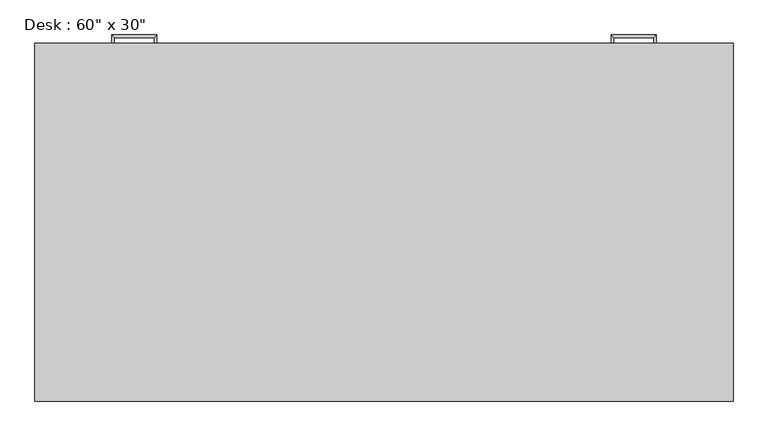
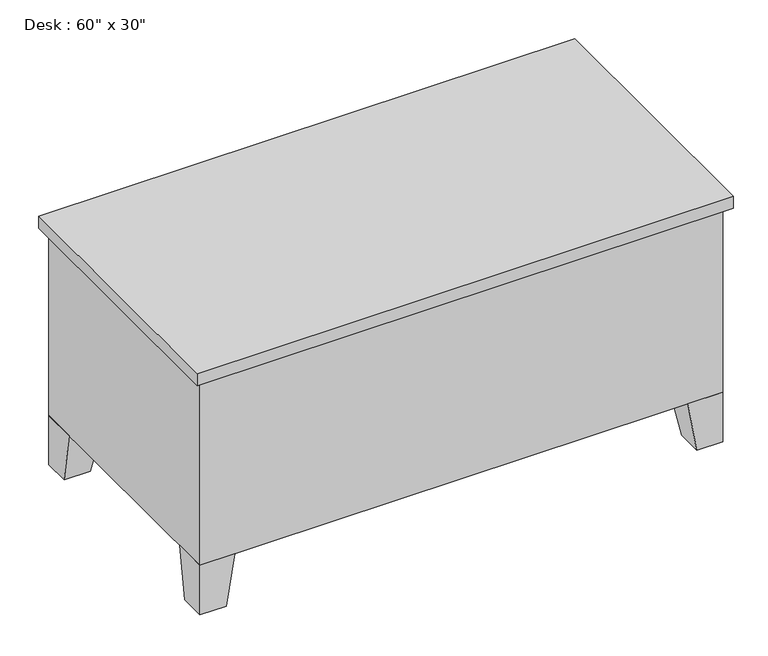
"""IFC4 building model written with IfcOpenShell, lengths in millimetres: furniture geometry."""

from ifc_helpers import new_model, si_unit, frame, origin, place, context, project, spatial, polyline, outline, extrude, faceted_brep, source, transform, mapped, element, save


def furniture_072f6425(model_context):
    return source(origin(), model_context, "Body", "SolidModel", [
        extrude(outline(polyline([(1504.95, 762.0), (1136.65, 762.0), (1136.65, 774.7), (1504.95, 774.7), (1504.95, 762.0)])), frame((0.0, 0.0, 603.25), z_axis=(0.0, 0.0, 1.0), x_axis=(1.0, 0.0, 0.0)), (0.0, 0.0, 1.0), 101.6),
        extrude(outline(polyline([(1504.95, 762.0), (1136.65, 762.0), (1136.65, 774.7), (1504.95, 774.7), (1504.95, 762.0)])), frame((0.0, 0.0, 171.45), z_axis=(0.0, 0.0, 1.0), x_axis=(1.0, 0.0, 0.0)), (0.0, 0.0, 1.0), 412.75),
        extrude(outline(polyline([(387.35, 762.0), (19.05, 762.0), (19.05, 774.7), (387.35, 774.7), (387.35, 762.0)])), frame((0.0, 0.0, 603.25), z_axis=(0.0, 0.0, 1.0), x_axis=(1.0, 0.0, 0.0)), (0.0, 0.0, 1.0), 101.6),
        extrude(outline(polyline([(387.35, 762.0), (19.05, 762.0), (19.05, 774.7), (387.35, 774.7), (387.35, 762.0)])), frame((0.0, 0.0, 171.45), z_axis=(0.0, 0.0, 1.0), x_axis=(1.0, 0.0, 0.0)), (0.0, 0.0, 1.0), 171.45),
        extrude(outline(polyline([(387.35, 762.0), (19.05, 762.0), (19.05, 774.7), (387.35, 774.7), (387.35, 762.0)])), frame((0.0, 0.0, 482.6), z_axis=(0.0, 0.0, 1.0), x_axis=(1.0, 0.0, 0.0)), (0.0, 0.0, 1.0), 101.6),
        extrude(outline(polyline([(387.35, 762.0), (19.05, 762.0), (19.05, 774.7), (387.35, 774.7), (387.35, 762.0)])), frame((0.0, 0.0, 361.95), z_axis=(0.0, 0.0, 1.0), x_axis=(1.0, 0.0, 0.0)), (0.0, 0.0, 1.0), 101.6),
        faceted_brep([(1422.4, 762.0, 152.4), (1422.4, 660.4, 152.4), (1524.0, 660.4, 152.4), (1524.0, 762.0, 152.4), (1447.8, 762.0, 0.0), (1524.0, 762.0, 0.0), (1524.0, 685.8, 0.0), (1447.8, 685.8, 0.0)], [[[0, 1, 2, 3]], [[4, 5, 6, 7]], [[4, 7, 1, 0]], [[7, 6, 2, 1]], [[6, 5, 3, 2]], [[5, 4, 0, 3]]]),
        faceted_brep([(1422.4, 0.0, 152.4), (1524.0, 0.0, 152.4), (1524.0, 101.6, 152.4), (1422.4, 101.6, 152.4), (1447.8, 0.0, 0.0), (1447.8, 76.2, 0.0), (1524.0, 76.2, 0.0), (1524.0, 0.0, 0.0)], [[[0, 1, 2, 3]], [[4, 5, 6, 7]], [[4, 7, 1, 0]], [[7, 6, 2, 1]], [[6, 5, 3, 2]], [[5, 4, 0, 3]]]),
        faceted_brep([(101.6, 0.0, 152.4), (101.6, 101.6, 152.4), (0.0, 101.6, 152.4), (0.0, 0.0, 152.4), (76.2, 0.0, 0.0), (0.0, 0.0, 0.0), (0.0, 76.2, 0.0), (76.2, 76.2, 0.0)], [[[0, 1, 2, 3]], [[4, 5, 6, 7]], [[4, 7, 1, 0]], [[7, 6, 2, 1]], [[6, 5, 3, 2]], [[5, 4, 0, 3]]]),
        faceted_brep([(101.6, 762.0, 152.4), (0.0, 762.0, 152.4), (0.0, 660.4, 152.4), (101.6, 660.4, 152.4), (76.2, 762.0, 0.0), (76.2, 685.8, 0.0), (0.0, 685.8, 0.0), (0.0, 762.0, 0.0)], [[[0, 1, 2, 3]], [[4, 5, 6, 7]], [[4, 7, 1, 0]], [[7, 6, 2, 1]], [[6, 5, 3, 2]], [[5, 4, 0, 3]]]),
        extrude(outline(polyline([(1543.05, 781.05), (1543.05, -19.05), (-19.05, -19.05), (-19.05, 781.05), (1543.05, 781.05)])), frame((0.0, 0.0, 723.9), z_axis=(0.0, 0.0, 1.0), x_axis=(1.0, 0.0, 0.0)), (0.0, 0.0, 1.0), 38.1),
        extrude(outline(polyline([(406.4, 762.0), (406.4, 50.8), (1117.6, 50.8), (1117.6, 762.0), (1524.0, 762.0), (1524.0, 0.0), (0.0, 0.0), (0.0, 762.0), (406.4, 762.0)])), frame((0.0, 0.0, 152.4), z_axis=(0.0, 0.0, 1.0), x_axis=(1.0, 0.0, 0.0)), (0.0, 0.0, 1.0), 571.5),
        faceted_brep([(1365.25, 774.7, 546.1), (1365.25, 774.7, 533.4), (1371.6, 774.7, 533.4), (1371.6, 774.7, 546.1), (1365.25, 793.75, 546.1), (1365.25, 793.75, 533.4), (1371.6, 800.1, 533.4), (1371.6, 800.1, 546.1), (1276.35, 793.75, 546.1), (1276.35, 793.75, 533.4), (1270.0, 800.1, 533.4), (1270.0, 800.1, 546.1), (1276.35, 774.7, 546.1), (1270.0, 774.7, 546.1), (1270.0, 774.7, 533.4), (1276.35, 774.7, 533.4)], [[[0, 1, 2, 3]], [[1, 0, 4, 5]], [[2, 1, 5, 6]], [[3, 2, 6, 7]], [[0, 3, 7, 4]], [[5, 4, 8, 9]], [[6, 5, 9, 10]], [[7, 6, 10, 11]], [[4, 7, 11, 8]], [[12, 13, 14, 15]], [[9, 8, 12, 15]], [[10, 9, 15, 14]], [[11, 10, 14, 13]], [[8, 11, 13, 12]]]),
        faceted_brep([(1365.25, 774.7, 666.75), (1365.25, 774.7, 654.05), (1371.6, 774.7, 654.05), (1371.6, 774.7, 666.75), (1365.25, 793.75, 666.75), (1365.25, 793.75, 654.05), (1371.6, 800.1, 654.05), (1371.6, 800.1, 666.75), (1276.35, 793.75, 666.75), (1276.35, 793.75, 654.05), (1270.0, 800.1, 654.05), (1270.0, 800.1, 666.75), (1276.35, 774.7, 666.75), (1270.0, 774.7, 666.75), (1270.0, 774.7, 654.05), (1276.35, 774.7, 654.05)], [[[0, 1, 2, 3]], [[1, 0, 4, 5]], [[2, 1, 5, 6]], [[3, 2, 6, 7]], [[0, 3, 7, 4]], [[5, 4, 8, 9]], [[6, 5, 9, 10]], [[7, 6, 10, 11]], [[4, 7, 11, 8]], [[12, 13, 14, 15]], [[9, 8, 12, 15]], [[10, 9, 15, 14]], [[11, 10, 14, 13]], [[8, 11, 13, 12]]]),
        faceted_brep([(158.75, 774.7, 304.8), (152.4, 774.7, 304.8), (152.4, 774.7, 292.1), (158.75, 774.7, 292.1), (158.75, 793.75, 304.8), (152.4, 800.1, 304.8), (152.4, 800.1, 292.1), (158.75, 793.75, 292.1), (247.65, 793.75, 304.8), (254.0, 800.1, 304.8), (254.0, 800.1, 292.1), (247.65, 793.75, 292.1), (247.65, 774.7, 304.8), (247.65, 774.7, 292.1), (254.0, 774.7, 292.1), (254.0, 774.7, 304.8)], [[[0, 1, 2, 3]], [[1, 0, 4, 5]], [[2, 1, 5, 6]], [[3, 2, 6, 7]], [[0, 3, 7, 4]], [[5, 4, 8, 9]], [[6, 5, 9, 10]], [[7, 6, 10, 11]], [[4, 7, 11, 8]], [[12, 13, 14, 15]], [[9, 8, 12, 15]], [[10, 9, 15, 14]], [[11, 10, 14, 13]], [[8, 11, 13, 12]]]),
        faceted_brep([(158.75, 774.7, 425.45), (152.4, 774.7, 425.45), (152.4, 774.7, 412.75), (158.75, 774.7, 412.75), (158.75, 793.75, 425.45), (152.4, 800.1, 425.45), (152.4, 800.1, 412.75), (158.75, 793.75, 412.75), (247.65, 793.75, 425.45), (254.0, 800.1, 425.45), (254.0, 800.1, 412.75), (247.65, 793.75, 412.75), (247.65, 774.7, 425.45), (247.65, 774.7, 412.75), (254.0, 774.7, 412.75), (254.0, 774.7, 425.45)], [[[0, 1, 2, 3]], [[1, 0, 4, 5]], [[2, 1, 5, 6]], [[3, 2, 6, 7]], [[0, 3, 7, 4]], [[5, 4, 8, 9]], [[6, 5, 9, 10]], [[7, 6, 10, 11]], [[4, 7, 11, 8]], [[12, 13, 14, 15]], [[9, 8, 12, 15]], [[10, 9, 15, 14]], [[11, 10, 14, 13]], [[8, 11, 13, 12]]]),
        faceted_brep([(158.75, 774.7, 546.1), (152.4, 774.7, 546.1), (152.4, 774.7, 533.4), (158.75, 774.7, 533.4), (158.75, 793.75, 546.1), (152.4, 800.1, 546.1), (152.4, 800.1, 533.4), (158.75, 793.75, 533.4), (247.65, 793.75, 546.1), (254.0, 800.1, 546.1), (254.0, 800.1, 533.4), (247.65, 793.75, 533.4), (247.65, 774.7, 546.1), (247.65, 774.7, 533.4), (254.0, 774.7, 533.4), (254.0, 774.7, 546.1)], [[[0, 1, 2, 3]], [[1, 0, 4, 5]], [[2, 1, 5, 6]], [[3, 2, 6, 7]], [[0, 3, 7, 4]], [[5, 4, 8, 9]], [[6, 5, 9, 10]], [[7, 6, 10, 11]], [[4, 7, 11, 8]], [[12, 13, 14, 15]], [[9, 8, 12, 15]], [[10, 9, 15, 14]], [[11, 10, 14, 13]], [[8, 11, 13, 12]]]),
        faceted_brep([(158.75, 774.7, 666.75), (152.4, 774.7, 666.75), (152.4, 774.7, 654.05), (158.75, 774.7, 654.05), (158.75, 793.75, 666.75), (152.4, 800.1, 666.75), (152.4, 800.1, 654.05), (158.75, 793.75, 654.05), (247.65, 793.75, 666.75), (254.0, 800.1, 666.75), (254.0, 800.1, 654.05), (247.65, 793.75, 654.05), (247.65, 774.7, 666.75), (247.65, 774.7, 654.05), (254.0, 774.7, 654.05), (254.0, 774.7, 666.75)], [[[0, 1, 2, 3]], [[1, 0, 4, 5]], [[2, 1, 5, 6]], [[3, 2, 6, 7]], [[0, 3, 7, 4]], [[5, 4, 8, 9]], [[6, 5, 9, 10]], [[7, 6, 10, 11]], [[4, 7, 11, 8]], [[12, 13, 14, 15]], [[9, 8, 12, 15]], [[10, 9, 15, 14]], [[11, 10, 14, 13]], [[8, 11, 13, 12]]]),
    ])


if __name__ == "__main__":
    model = new_model("IFC4")
    model_context = context("Model", 3, world=origin())
    ifc_project = project(units=[si_unit("LENGTHUNIT", "METRE", prefix="MILLI")], contexts=[model_context])
    site = spatial("IfcSite", under=ifc_project)
    building = spatial("IfcBuilding", under=site)
    placement = place(None, origin())
    furniture_shape = furniture_072f6425(model_context)
    element("IfcFurniture", 1, ObjectType="Desk : 60\" x 30\"", at=placement, inside=building, context=model_context, shape_type="MappedRepresentation", body=[
        mapped(furniture_shape, transform((0.0, 0.0, 0.0), x_axis=(1.0, 0.0, 0.0), y_axis=(0.0, 1.0, 0.0), z_axis=(0.0, 0.0, 1.0))),
    ])
    save(model, "model.ifc")

# Revit data of these elements
# Type "Desk : 60\" x 30\""
#   Assembly Code = "E2020200"
#   Depth = 2' - 6"
#   Height = 2' - 6"
#   Leg Height = 0' - 6"
#   Width = 5' - 0"
#   Body Material = Laminate, Ivory, Matte
#   Handle/Leg Material = Steel, Chrome Plated
#   Top Material = Cherry
# Element 1 (IfcFurniture, "Desk : 60\" x 30\"")
#   Materials on its faces: "Steel, Chrome Plated", "Laminate, Ivory, Matte", "Cherry"
# Materials
#   "Laminate, Ivory, Matte": class "Plastic", colour RGB 247 247 239, transparency 0, Description = "Plastic Laminate - Ivory, Matte", Cost = 0
#   "Steel, Chrome Plated": class "Metal", colour RGB 17 17 17, transparency 0, Description = "Chromiuim plated steel", Cost = 0
#   "Cherry": class "Wood", colour RGB 226 177 128, transparency 0, Description = "Prunus Serotina", Cost = 0
